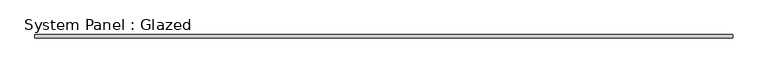
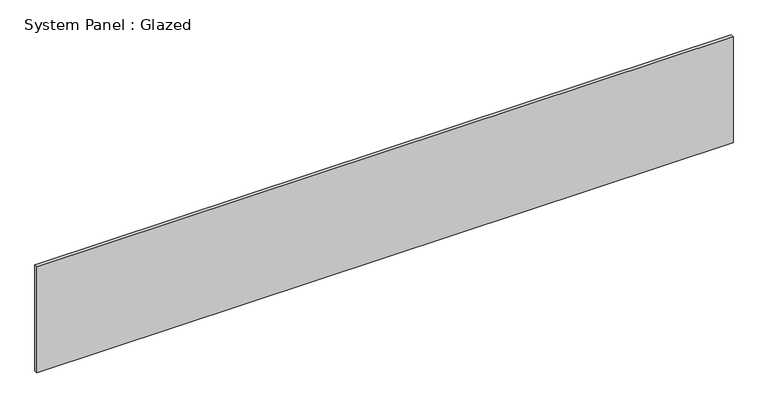
"""IFC4 building model written with IfcOpenShell, lengths in millimetres: plate geometry, System Panel : Glazed."""

from ifc_helpers import new_model, si_unit, origin, origin_with_axes, place, context, project, spatial, polyline, outline, extrude, source, transform, mapped, element, save


def system_panel_glazed_62b5ff2e(model_context):
    return source(origin(), model_context, "Body", "SweptSolid", [
        extrude(outline(polyline([(2711.45, 19.05), (-2711.45, 19.05), (-2711.45, 44.45), (2711.45, 44.45), (2711.45, 19.05)])), origin_with_axes(), (0.0, 0.0, 1.0), 870.961214),
    ])


if __name__ == "__main__":
    model = new_model("IFC4")
    model_context = context("Model", 3, world=origin())
    ifc_project = project(units=[si_unit("LENGTHUNIT", "METRE", prefix="MILLI")], contexts=[model_context])
    site = spatial("IfcSite", under=ifc_project)
    building = spatial("IfcBuilding", under=site)
    placement = place(None, origin())
    system_panel_glazed_shape = system_panel_glazed_62b5ff2e(model_context)
    element("IfcPlate", 1, ObjectType="System Panel : Glazed", at=placement, inside=building, context=model_context, shape_type="MappedRepresentation", body=[
        mapped(system_panel_glazed_shape, transform((0.0, 0.0, 0.0), x_axis=(1.0, 0.0, 0.0), y_axis=(0.0, 1.0, 0.0), z_axis=(0.0, 0.0, 1.0))),
    ])
    save(model, "model.ifc")

# Revit data of these elements
# Type "System Panel : Glazed"
#   Construction Type Id = "GSP4R"
#   Analytic Construction = "1/8 in Pilkington single glazing"
#   Visual Light Transmittance = 0.9
#   Solar Heat Gain Coefficient = 0.86
#   Heat Transfer Coefficient (U) = 1.18115 BTU/(h·ft²·°F)
#   Define Thermal Properties by = 1
# Element 1 (IfcPlate, "System Panel : Glazed")
#   Materials on its faces: "Glass"
# Materials
#   "Glass": class "Glass", colour RGB 0 128 192, transparency 0.75, Description = "Soda Lime Glass", Cost = 0
